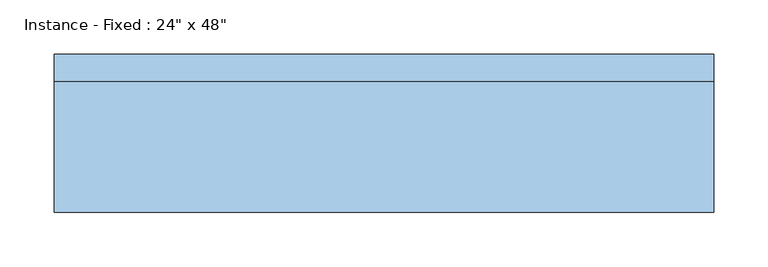
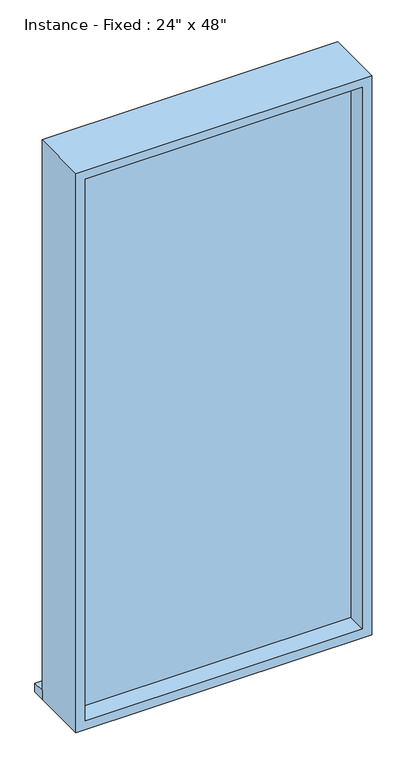
"""IFC4 building model written with IfcOpenShell, lengths in millimetres: window geometry."""

from ifc_helpers import new_model, si_unit, frame, origin, place, context, project, spatial, polyline, outline, extrude, source, transform, mapped, element, save


def window_20ff4747(model_context):
    return source(origin(), model_context, "Body", "SweptSolid", [
        extrude(outline(polyline([(-342.9, 127.0), (266.7, 127.0), (266.7, 101.6), (-342.9, 101.6), (-342.9, 127.0)])), frame((0.0, 0.0, 914.4), z_axis=(0.0, 0.0, 1.0), x_axis=(1.0, 0.0, 0.0)), (0.0, 0.0, 1.0), 19.05),
        extrude(outline(polyline([(247.65, 22.225), (-323.85, 22.225), (-323.85, 34.925), (247.65, 34.925), (247.65, 22.225)])), frame((0.0, 0.0, 933.45), z_axis=(0.0, 0.0, 1.0), x_axis=(1.0, 0.0, 0.0)), (0.0, 0.0, 1.0), 1181.1),
        extrude(outline(polyline([(2133.6, 266.7), (2133.6, -342.9), (914.4, -342.9), (914.4, 266.7), (2133.6, 266.7)]), holes=[polyline([(2114.55, 247.65), (933.45, 247.65), (933.45, -323.85), (2114.55, -323.85), (2114.55, 247.65)])]), frame((0.0, -19.05, 0.0), z_axis=(0.0, 1.0, 0.0), x_axis=(0.0, 0.0, 1.0)), (0.0, 0.0, 1.0), 120.65),
    ])


if __name__ == "__main__":
    model = new_model("IFC4")
    model_context = context("Model", 3, world=origin())
    ifc_project = project(units=[si_unit("LENGTHUNIT", "METRE", prefix="MILLI")], contexts=[model_context])
    site = spatial("IfcSite", under=ifc_project)
    building = spatial("IfcBuilding", under=site)
    placement = place(None, origin())
    window_shape = window_20ff4747(model_context)
    element("IfcWindow", 1, ObjectType="Instance - Fixed : 24\" x 48\"", at=placement, inside=building, context=model_context, shape_type="MappedRepresentation", body=[
        mapped(window_shape, transform((0.0, 0.0, 0.0), x_axis=(1.0, 0.0, 0.0), y_axis=(0.0, 1.0, 0.0), z_axis=(0.0, 0.0, 1.0))),
    ])
    save(model, "model.ifc")

# Revit data of these elements
# Type "Instance - Fixed : 24\" x 48\""
#   Type Mark = "11"
#   Construction Type Id = "GSP4R"
#   Assembly Code = "B2020100"
#   Analytic Construction = "1/8 in Pilkington single glazing"
#   Visual Light Transmittance = 0.9
#   Thermal Resistance (R) = 0.8466 (h·ft²·°F)/BTU
#   Solar Heat Gain Coefficient = 0.86
#   Heat Transfer Coefficient (U) = 1.1812 BTU/(h·ft²·°F)
#   Height [instance default] = 4' - 0"
#   Default Sill Height = 3' - 0"
#   Width [instance default] = 2' - 0"
#   Window Inset = 0' - 2"
#   Define Thermal Properties by = 1
#   Glass Pane Material = Glass
#   Sash Material = Iron, Ductile
#   Wall Closure = (empty or 0)
# Element 1 (IfcWindow, "Instance - Fixed : 24\" x 48\"")
#   Materials on its faces: "Iron, Ductile", "Glass"
# Materials
#   "Glass": class "Glass", colour RGB 0 128 192, transparency 0.75, Description = "Soda Lime Glass", Cost = 0
#   "Iron, Ductile": class "Metal", colour RGB 0 0 0, transparency 0, Description = "Ductile cast iron", Cost = 0
